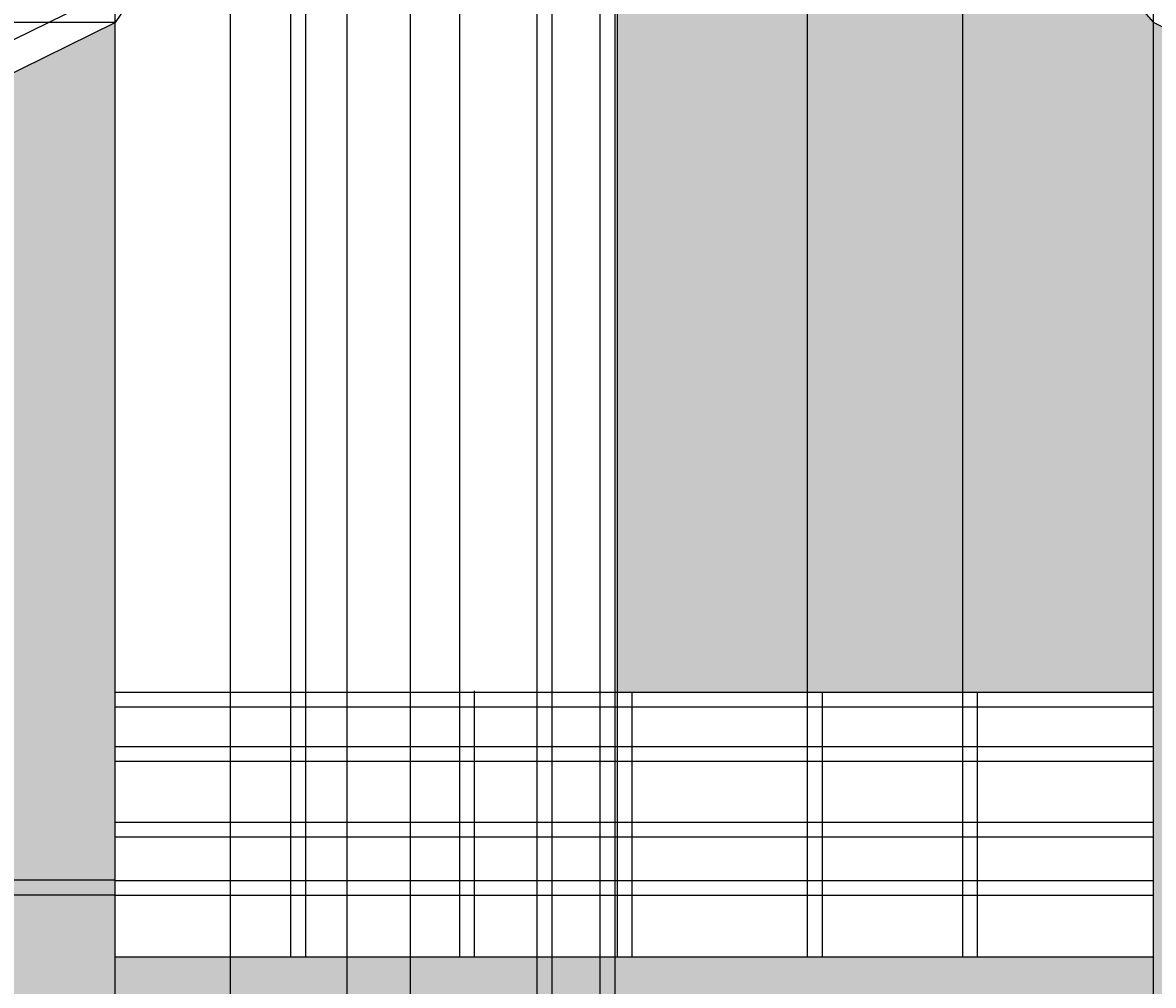
# Model space of a CAD drawing. Units: inches. Extents: x 36 to 594, y 79 to 831.
# Tile 23 of 30: x 189 to 342, y 590 to 721. Entities that reach past the tile are written whole.
import ezdxf

# ---------------------------------------------------------------- set-up
doc = ezdxf.new("R2010")
doc.units = ezdxf.units.IN
doc.header["$MEASUREMENT"] = 0
for name, color, linetype, lineweight in [('A-ANNO-DIMS', 2, 'Continuous', 18), ('A-ELEV', 7, 'Continuous', 25), ('A-ELEV-PATT', 8, 'Continuous', 13)]:
    doc.layers.add(name, color=color, linetype=linetype, lineweight=lineweight)
doc.styles.get("Standard").update_dxf_attribs({"font": 'arial.ttf'})
doc.dimstyles.get("Standard").update_dxf_attribs({"dimtxt": 0.8125, "dimasz": 0.18, "dimexe": 0.18, "dimexo": 0.0625, "dimgap": 0.09, "dimtad": 0, "dimtih": 1, "dimtoh": 1, "dimdec": 4, "dimzin": 0, "dimdsep": 46, "dimlunit": 4, "dimtxsty": 'Standard', "dimcen": 0.09, "dimadec": 0, "dimazin": 0, "dimtfac": 1, "dimtdec": 4, "dimtofl": 0, "dimtmove": 0, "dimatfit": 3, "dimfxl": 1, "dimtolj": 1, "dimtzin": 0, "dimarcsym": 0})

# ---------------------------------------------------------------- blocks, each defined once
blk = doc.blocks.new('*D14')
at = {"layer": 'A-ANNO-DIMS', "color": 0, "lineweight": -2, "transparency": 16777216}
for p, q in [((177.52, 594.27), (177.52, 830.73)), ((177.7, 830.55), (187.69, 830.55)), ((201.24, 830.55), (191.25, 830.55)), ((201.42, 720.66), (201.42, 830.73))]:
    blk.add_line(p, q, dxfattribs=at)
at = {"layer": 'A-ANNO-DIMS', "color": 0, "transparency": 16777216}
for points in [[(177.7, 830.58), (177.7, 830.52), (177.52, 830.55)], [(201.24, 830.58), (201.24, 830.52), (201.42, 830.55)]]:
    blk.add_solid(points, dxfattribs=at)
at = {"layer": 'Defpoints', "color": 0, "transparency": 16777216}
for p in [(201.42, 830.55), (201.42, 720.59), (177.52, 594.21)]:
    blk.add_point(p, dxfattribs=at)
at = {"layer": 'A-ANNO-DIMS', "color": 0, "transparency": 16777216, "insert": (189.47, 830.55), "char_height": 0.812, "attachment_point": 5}
blk.add_mtext('\\A1;23.894', dxfattribs=at)
blk = doc.blocks.new('*D28')
at = {"layer": 'A-ANNO-DIMS', "color": 0, "lineweight": -2, "transparency": 16777216}
for p, q in [((269.3, 796.05), (37.49, 796.05)), ((37.67, 795.87), (37.67, 455.63)), ((37.67, 114.39), (37.67, 454.62)), ((94.8, 114.21), (37.49, 114.21))]:
    blk.add_line(p, q, dxfattribs=at)
at = {"layer": 'A-ANNO-DIMS', "color": 0, "transparency": 16777216}
for points in [[(37.64, 795.87), (37.7, 795.87), (37.67, 796.05)], [(37.64, 114.39), (37.7, 114.39), (37.67, 114.21)]]:
    blk.add_solid(points, dxfattribs=at)
at = {"layer": 'Defpoints', "color": 0, "transparency": 16777216}
for p in [(37.67, 796.05), (269.36, 796.05), (94.87, 114.21)]:
    blk.add_point(p, dxfattribs=at)
at = {"layer": 'A-ANNO-DIMS', "color": 0, "transparency": 16777216, "insert": (37.67, 455.13), "char_height": 0.812, "attachment_point": 5}
blk.add_mtext('\\A1;681.8', dxfattribs=at)
blk = doc.blocks.new('*D37')
at = {"layer": 'A-ANNO-DIMS', "color": 0, "lineweight": -2, "transparency": 16777216}
for p, q in [((330.04, 735.34), (592.85, 735.34)), ((592.67, 735.16), (592.67, 702.28)), ((592.67, 668.39), (592.67, 701.27)), ((448.45, 668.21), (592.85, 668.21))]:
    blk.add_line(p, q, dxfattribs=at)
at = {"layer": 'A-ANNO-DIMS', "color": 0, "transparency": 16777216}
for points in [[(592.64, 735.16), (592.7, 735.16), (592.67, 735.34)], [(592.64, 668.39), (592.7, 668.39), (592.67, 668.21)]]:
    blk.add_solid(points, dxfattribs=at)
at = {"layer": 'Defpoints', "color": 0, "transparency": 16777216}
for p in [(329.98, 735.34), (592.67, 735.34), (448.39, 668.21)]:
    blk.add_point(p, dxfattribs=at)
at = {"layer": 'A-ANNO-DIMS', "color": 0, "transparency": 16777216, "insert": (592.67, 701.77), "char_height": 0.812, "attachment_point": 5}
blk.add_mtext('\\A1;67.12', dxfattribs=at)
blk = doc.blocks.new('*D48')
at = {"layer": 'A-ANNO-DIMS', "color": 0, "lineweight": -2, "transparency": 16777216}
for p, q in [((201.36, 720.59), (37.49, 720.59)), ((37.67, 720.41), (37.67, 694.91)), ((37.67, 668.39), (37.67, 693.9)), ((94.8, 668.21), (37.49, 668.21))]:
    blk.add_line(p, q, dxfattribs=at)
at = {"layer": 'A-ANNO-DIMS', "color": 0, "transparency": 16777216}
for points in [[(37.64, 720.41), (37.7, 720.41), (37.67, 720.59)], [(37.64, 668.39), (37.7, 668.39), (37.67, 668.21)]]:
    blk.add_solid(points, dxfattribs=at)
at = {"layer": 'Defpoints', "color": 0, "transparency": 16777216}
for p in [(37.67, 720.59), (201.42, 720.59), (94.87, 668.21)]:
    blk.add_point(p, dxfattribs=at)
at = {"layer": 'A-ANNO-DIMS', "color": 0, "transparency": 16777216, "insert": (37.67, 694.4), "char_height": 0.812, "attachment_point": 5}
blk.add_mtext('\\A1;52.38', dxfattribs=at)
blk = doc.blocks.new('*D61')
at = {"layer": 'A-ANNO-DIMS', "color": 0, "lineweight": -2, "transparency": 16777216}
for p, q in [((156.41, 264.68), (156.41, 830.73)), ((156.59, 830.55), (185.26, 830.55)), ((216.85, 830.55), (188.18, 830.55)), ((217.03, 286.24), (217.03, 830.73))]:
    blk.add_line(p, q, dxfattribs=at)
at = {"layer": 'A-ANNO-DIMS', "color": 0, "transparency": 16777216}
for points in [[(156.59, 830.58), (156.59, 830.52), (156.41, 830.55)], [(216.85, 830.58), (216.85, 830.52), (217.03, 830.55)]]:
    blk.add_solid(points, dxfattribs=at)
at = {"layer": 'Defpoints', "color": 0, "transparency": 16777216}
for p in [(217.03, 830.55), (217.03, 286.18), (156.41, 264.62)]:
    blk.add_point(p, dxfattribs=at)
at = {"layer": 'A-ANNO-DIMS', "color": 0, "transparency": 16777216, "insert": (186.72, 830.55), "char_height": 0.812, "attachment_point": 5}
blk.add_mtext('\\A1;60.62', dxfattribs=at)
blk = doc.blocks.new('*D92')
at = {"layer": 'A-ANNO-DIMS', "color": 0, "lineweight": -2, "transparency": 16777216}
for p, q in [((201.42, 475.48), (201.42, 830.73)), ((201.6, 830.55), (215.98, 830.55)), ((232.64, 830.55), (218.26, 830.55)), ((232.82, 524.67), (232.82, 830.73))]:
    blk.add_line(p, q, dxfattribs=at)
at = {"layer": 'A-ANNO-DIMS', "color": 0, "transparency": 16777216}
for points in [[(201.6, 830.58), (201.6, 830.52), (201.42, 830.55)], [(232.64, 830.58), (232.64, 830.52), (232.82, 830.55)]]:
    blk.add_solid(points, dxfattribs=at)
at = {"layer": 'Defpoints', "color": 0, "transparency": 16777216}
for p in [(232.82, 830.55), (232.82, 524.6), (201.42, 475.41)]:
    blk.add_point(p, dxfattribs=at)
at = {"layer": 'A-ANNO-DIMS', "color": 0, "transparency": 16777216, "insert": (217.12, 830.55), "char_height": 0.812, "attachment_point": 5}
blk.add_mtext('\\A1;31.4', dxfattribs=at)
blk = doc.blocks.new('*D93')
at = {"layer": 'A-ANNO-DIMS', "color": 0, "lineweight": -2, "transparency": 16777216}
for p, q in [((232.82, 524.67), (232.82, 830.73)), ((233, 830.55), (243.88, 830.55)), ((258.33, 830.55), (247.45, 830.55)), ((258.51, 524.67), (258.51, 830.73))]:
    blk.add_line(p, q, dxfattribs=at)
at = {"layer": 'A-ANNO-DIMS', "color": 0, "transparency": 16777216}
for points in [[(233, 830.58), (233, 830.52), (232.82, 830.55)], [(258.33, 830.58), (258.33, 830.52), (258.51, 830.55)]]:
    blk.add_solid(points, dxfattribs=at)
at = {"layer": 'Defpoints', "color": 0, "transparency": 16777216}
for p in [(258.51, 830.55), (232.82, 524.6), (258.51, 524.6)]:
    blk.add_point(p, dxfattribs=at)
at = {"layer": 'A-ANNO-DIMS', "color": 0, "transparency": 16777216, "insert": (245.66, 830.55), "char_height": 0.812, "attachment_point": 5}
blk.add_mtext('\\A1;25.684', dxfattribs=at)
blk = doc.blocks.new('*D94')
at = {"layer": 'A-ANNO-DIMS', "color": 0, "lineweight": -2, "transparency": 16777216}
for p, q in [((258.51, 524.67), (258.51, 830.73)), ((258.69, 830.55), (259.15, 830.55)), ((260.33, 830.55), (259.86, 830.55)), ((260.51, 524.67), (260.51, 830.73))]:
    blk.add_line(p, q, dxfattribs=at)
at = {"layer": 'A-ANNO-DIMS', "color": 0, "transparency": 16777216}
for points in [[(258.69, 830.58), (258.69, 830.52), (258.51, 830.55)], [(260.33, 830.58), (260.33, 830.52), (260.51, 830.55)]]:
    blk.add_solid(points, dxfattribs=at)
at = {"layer": 'Defpoints', "color": 0, "transparency": 16777216}
for p in [(260.51, 830.55), (258.51, 524.6), (260.51, 524.6)]:
    blk.add_point(p, dxfattribs=at)
at = {"layer": 'A-ANNO-DIMS', "color": 0, "transparency": 16777216, "insert": (259.51, 830.55), "char_height": 0.812, "attachment_point": 5}
blk.add_mtext('\\A1;2', dxfattribs=at)
blk = doc.blocks.new('*D95')
at = {"layer": 'A-ANNO-DIMS', "color": 0, "lineweight": -2, "transparency": 16777216}
for p, q in [((260.51, 524.67), (260.51, 830.73)), ((260.69, 830.55), (299.71, 830.55)), ((341.66, 830.55), (302.63, 830.55)), ((341.84, 524.67), (341.84, 830.73))]:
    blk.add_line(p, q, dxfattribs=at)
at = {"layer": 'A-ANNO-DIMS', "color": 0, "transparency": 16777216}
for points in [[(260.69, 830.58), (260.69, 830.52), (260.51, 830.55)], [(341.66, 830.58), (341.66, 830.52), (341.84, 830.55)]]:
    blk.add_solid(points, dxfattribs=at)
at = {"layer": 'Defpoints', "color": 0, "transparency": 16777216}
for p in [(341.84, 830.55), (260.51, 524.6), (341.84, 524.6)]:
    blk.add_point(p, dxfattribs=at)
at = {"layer": 'A-ANNO-DIMS', "color": 0, "transparency": 16777216, "insert": (301.17, 830.55), "char_height": 0.812, "attachment_point": 5}
blk.add_mtext('\\A1;81.33', dxfattribs=at)
blk = doc.blocks.new('*D105')
at = {"layer": 'A-ANNO-DIMS', "color": 0, "lineweight": -2, "transparency": 16777216}
for p, q in [((241.36, 404.34), (241.36, 830.73)), ((241.54, 830.55), (252.42, 830.55)), ((266.86, 830.55), (255.98, 830.55)), ((267.04, 404.34), (267.04, 830.73))]:
    blk.add_line(p, q, dxfattribs=at)
at = {"layer": 'A-ANNO-DIMS', "color": 0, "transparency": 16777216}
for points in [[(241.54, 830.58), (241.54, 830.52), (241.36, 830.55)], [(266.86, 830.58), (266.86, 830.52), (267.04, 830.55)]]:
    blk.add_solid(points, dxfattribs=at)
at = {"layer": 'Defpoints', "color": 0, "transparency": 16777216}
for p in [(267.04, 830.55), (241.36, 404.27), (267.04, 404.27)]:
    blk.add_point(p, dxfattribs=at)
at = {"layer": 'A-ANNO-DIMS', "color": 0, "transparency": 16777216, "insert": (254.2, 830.55), "char_height": 0.812, "attachment_point": 5}
blk.add_mtext('\\A1;25.684', dxfattribs=at)
blk = doc.blocks.new('*D106')
at = {"layer": 'A-ANNO-DIMS', "color": 0, "lineweight": -2, "transparency": 16777216}
for p, q in [((267.04, 404.34), (267.04, 830.73)), ((267.22, 830.55), (267.68, 830.55)), ((268.86, 830.55), (268.4, 830.55)), ((269.04, 404.34), (269.04, 830.73))]:
    blk.add_line(p, q, dxfattribs=at)
at = {"layer": 'A-ANNO-DIMS', "color": 0, "transparency": 16777216}
for points in [[(267.22, 830.58), (267.22, 830.52), (267.04, 830.55)], [(268.86, 830.58), (268.86, 830.52), (269.04, 830.55)]]:
    blk.add_solid(points, dxfattribs=at)
at = {"layer": 'Defpoints', "color": 0, "transparency": 16777216}
for p in [(269.04, 830.55), (267.04, 404.27), (269.04, 404.27)]:
    blk.add_point(p, dxfattribs=at)
at = {"layer": 'A-ANNO-DIMS', "color": 0, "transparency": 16777216, "insert": (268.04, 830.55), "char_height": 0.812, "attachment_point": 5}
blk.add_mtext('\\A1;2', dxfattribs=at)
blk = doc.blocks.new('*D107')
at = {"layer": 'A-ANNO-DIMS', "color": 0, "lineweight": -2, "transparency": 16777216}
for p, q in [((269.04, 404.34), (269.04, 830.73)), ((269.22, 830.55), (310.99, 830.55)), ((355.68, 830.55), (313.91, 830.55)), ((355.86, 404.34), (355.86, 830.73))]:
    blk.add_line(p, q, dxfattribs=at)
at = {"layer": 'A-ANNO-DIMS', "color": 0, "transparency": 16777216}
for points in [[(269.22, 830.58), (269.22, 830.52), (269.04, 830.55)], [(355.68, 830.58), (355.68, 830.52), (355.86, 830.55)]]:
    blk.add_solid(points, dxfattribs=at)
at = {"layer": 'Defpoints', "color": 0, "transparency": 16777216}
for p in [(355.86, 830.55), (269.04, 404.27), (355.86, 404.27)]:
    blk.add_point(p, dxfattribs=at)
at = {"layer": 'A-ANNO-DIMS', "color": 0, "transparency": 16777216, "insert": (312.45, 830.55), "char_height": 0.812, "attachment_point": 5}
blk.add_mtext('\\A1;86.82', dxfattribs=at)
blk = doc.blocks.new('*D122')
at = {"layer": 'A-ANNO-DIMS', "color": 0, "lineweight": -2, "transparency": 16777216}
for p, q in [((201.36, 604.57), (37.49, 604.57)), ((37.67, 604.39), (37.67, 604.06)), ((201.36, 602.57), (37.49, 602.57)), ((37.67, 602.75), (37.67, 603.07))]:
    blk.add_line(p, q, dxfattribs=at)
at = {"layer": 'A-ANNO-DIMS', "color": 0, "transparency": 16777216}
for points in [[(37.64, 604.39), (37.7, 604.39), (37.67, 604.57)], [(37.64, 602.75), (37.7, 602.75), (37.67, 602.57)]]:
    blk.add_solid(points, dxfattribs=at)
at = {"layer": 'Defpoints', "color": 0, "transparency": 16777216}
for p in [(37.67, 604.57), (201.42, 604.57), (201.42, 602.57)]:
    blk.add_point(p, dxfattribs=at)
at = {"layer": 'A-ANNO-DIMS', "color": 0, "transparency": 16777216, "insert": (37.67, 603.57), "char_height": 0.812, "attachment_point": 5}
blk.add_mtext('\\A1;2', dxfattribs=at)
blk = doc.blocks.new('*D123')
at = {"layer": 'A-ANNO-DIMS', "color": 0, "lineweight": -2, "transparency": 16777216}
for p, q in [((201.42, 630.1), (201.42, 830.73)), ((201.6, 830.55), (211.52, 830.55)), ((225.01, 830.55), (215.09, 830.55)), ((225.19, 630.1), (225.19, 830.73))]:
    blk.add_line(p, q, dxfattribs=at)
at = {"layer": 'A-ANNO-DIMS', "color": 0, "transparency": 16777216}
for points in [[(201.6, 830.58), (201.6, 830.52), (201.42, 830.55)], [(225.01, 830.58), (225.01, 830.52), (225.19, 830.55)]]:
    blk.add_solid(points, dxfattribs=at)
at = {"layer": 'Defpoints', "color": 0, "transparency": 16777216}
for p in [(225.19, 830.55), (201.42, 630.04), (225.19, 630.04)]:
    blk.add_point(p, dxfattribs=at)
at = {"layer": 'A-ANNO-DIMS', "color": 0, "transparency": 16777216, "insert": (213.31, 830.55), "char_height": 0.812, "attachment_point": 5}
blk.add_mtext('\\A1;23.773', dxfattribs=at)
blk = doc.blocks.new('*D124')
at = {"layer": 'A-ANNO-DIMS', "color": 0, "lineweight": -2, "transparency": 16777216}
for p, q in [((225.19, 630.1), (225.19, 830.73)), ((225.37, 830.55), (225.83, 830.55)), ((227.01, 830.55), (226.55, 830.55)), ((227.19, 630.1), (227.19, 830.73))]:
    blk.add_line(p, q, dxfattribs=at)
at = {"layer": 'A-ANNO-DIMS', "color": 0, "transparency": 16777216}
for points in [[(225.37, 830.58), (225.37, 830.52), (225.19, 830.55)], [(227.01, 830.58), (227.01, 830.52), (227.19, 830.55)]]:
    blk.add_solid(points, dxfattribs=at)
at = {"layer": 'Defpoints', "color": 0, "transparency": 16777216}
for p in [(227.19, 830.55), (225.19, 630.04), (227.19, 630.04)]:
    blk.add_point(p, dxfattribs=at)
at = {"layer": 'A-ANNO-DIMS', "color": 0, "transparency": 16777216, "insert": (226.19, 830.55), "char_height": 0.812, "attachment_point": 5}
blk.add_mtext('\\A1;2', dxfattribs=at)
blk = doc.blocks.new('*D125')
at = {"layer": 'A-ANNO-DIMS', "color": 0, "lineweight": -2, "transparency": 16777216}
for p, q in [((227.19, 630.1), (227.19, 830.73)), ((227.37, 830.55), (236.14, 830.55)), ((247.84, 830.55), (239.07, 830.55)), ((248.02, 630.27), (248.02, 830.73))]:
    blk.add_line(p, q, dxfattribs=at)
at = {"layer": 'A-ANNO-DIMS', "color": 0, "transparency": 16777216}
for points in [[(227.37, 830.58), (227.37, 830.52), (227.19, 830.55)], [(247.84, 830.58), (247.84, 830.52), (248.02, 830.55)]]:
    blk.add_solid(points, dxfattribs=at)
at = {"layer": 'Defpoints', "color": 0, "transparency": 16777216}
for p in [(248.02, 830.55), (248.02, 630.21), (227.19, 630.04)]:
    blk.add_point(p, dxfattribs=at)
at = {"layer": 'A-ANNO-DIMS', "color": 0, "transparency": 16777216, "insert": (237.61, 830.55), "char_height": 0.812, "attachment_point": 5}
blk.add_mtext('\\A1;20.83', dxfattribs=at)
blk = doc.blocks.new('*D126')
at = {"layer": 'A-ANNO-DIMS', "color": 0, "lineweight": -2, "transparency": 16777216}
for p, q in [((248.02, 630.27), (248.02, 830.73)), ((248.2, 830.55), (256.91, 830.55)), ((269.18, 830.55), (260.47, 830.55)), ((269.36, 630.1), (269.36, 830.73))]:
    blk.add_line(p, q, dxfattribs=at)
at = {"layer": 'A-ANNO-DIMS', "color": 0, "transparency": 16777216}
for points in [[(248.2, 830.58), (248.2, 830.52), (248.02, 830.55)], [(269.18, 830.58), (269.18, 830.52), (269.36, 830.55)]]:
    blk.add_solid(points, dxfattribs=at)
at = {"layer": 'Defpoints', "color": 0, "transparency": 16777216}
for p in [(269.36, 830.55), (248.02, 630.21), (269.36, 630.04)]:
    blk.add_point(p, dxfattribs=at)
at = {"layer": 'A-ANNO-DIMS', "color": 0, "transparency": 16777216, "insert": (258.69, 830.55), "char_height": 0.812, "attachment_point": 5}
blk.add_mtext('\\A1;21.338', dxfattribs=at)
blk = doc.blocks.new('*D127')
at = {"layer": 'A-ANNO-DIMS', "color": 0, "lineweight": -2, "transparency": 16777216}
for p, q in [((269.36, 630.1), (269.36, 830.73)), ((269.54, 830.55), (280.75, 830.55)), ((294.9, 830.55), (283.68, 830.55)), ((295.08, 630.1), (295.08, 830.73))]:
    blk.add_line(p, q, dxfattribs=at)
at = {"layer": 'A-ANNO-DIMS', "color": 0, "transparency": 16777216}
for points in [[(269.54, 830.58), (269.54, 830.52), (269.36, 830.55)], [(294.9, 830.58), (294.9, 830.52), (295.08, 830.55)]]:
    blk.add_solid(points, dxfattribs=at)
at = {"layer": 'Defpoints', "color": 0, "transparency": 16777216}
for p in [(295.08, 830.55), (269.36, 630.04), (295.08, 630.04)]:
    blk.add_point(p, dxfattribs=at)
at = {"layer": 'A-ANNO-DIMS', "color": 0, "transparency": 16777216, "insert": (282.22, 830.55), "char_height": 0.812, "attachment_point": 5}
blk.add_mtext('\\A1;25.72', dxfattribs=at)
blk = doc.blocks.new('*D128')
at = {"layer": 'A-ANNO-DIMS', "color": 0, "lineweight": -2, "transparency": 16777216}
for p, q in [((295.08, 630.1), (295.08, 830.73)), ((295.26, 830.55), (303.78, 830.55)), ((315.87, 830.55), (307.35, 830.55)), ((316.05, 630.1), (316.05, 830.73))]:
    blk.add_line(p, q, dxfattribs=at)
at = {"layer": 'A-ANNO-DIMS', "color": 0, "transparency": 16777216}
for points in [[(295.26, 830.58), (295.26, 830.52), (295.08, 830.55)], [(315.87, 830.58), (315.87, 830.52), (316.05, 830.55)]]:
    blk.add_solid(points, dxfattribs=at)
at = {"layer": 'Defpoints', "color": 0, "transparency": 16777216}
for p in [(316.05, 830.55), (295.08, 630.04), (316.05, 630.04)]:
    blk.add_point(p, dxfattribs=at)
at = {"layer": 'A-ANNO-DIMS', "color": 0, "transparency": 16777216, "insert": (305.56, 830.55), "char_height": 0.812, "attachment_point": 5}
blk.add_mtext('\\A1;20.974', dxfattribs=at)
blk = doc.blocks.new('*D129')
at = {"layer": 'A-ANNO-DIMS', "color": 0, "lineweight": -2, "transparency": 16777216}
for p, q in [((316.05, 630.1), (316.05, 830.73)), ((316.23, 830.55), (327.16, 830.55)), ((341.66, 830.55), (330.73, 830.55)), ((341.84, 630.1), (341.84, 830.73))]:
    blk.add_line(p, q, dxfattribs=at)
at = {"layer": 'A-ANNO-DIMS', "color": 0, "transparency": 16777216}
for points in [[(316.23, 830.58), (316.23, 830.52), (316.05, 830.55)], [(341.66, 830.58), (341.66, 830.52), (341.84, 830.55)]]:
    blk.add_solid(points, dxfattribs=at)
at = {"layer": 'Defpoints', "color": 0, "transparency": 16777216}
for p in [(341.84, 830.55), (316.05, 630.04), (341.84, 630.04)]:
    blk.add_point(p, dxfattribs=at)
at = {"layer": 'A-ANNO-DIMS', "color": 0, "transparency": 16777216, "insert": (328.94, 830.55), "char_height": 0.812, "attachment_point": 5}
blk.add_mtext('\\A1;25.785', dxfattribs=at)

msp = doc.modelspace()

# ---------------------------------------------------------------- hatches: boundary and pattern name
at = {"layer": 'A-ELEV-PATT'}
h = msp.add_hatch(color=256, dxfattribs=at)
h.dxf.hatch_style = 1
h.paths.add_polyline_path([(398.0873, 796.0465), (269.3592, 796.0465), (269.3592, 770.1455), (397.8159, 770.1455)])
h.paths.add_polyline_path([(397.7518, 764.0341), (269.3592, 764.0341), (269.3592, 630.0394), (341.8367, 630.0394), (341.8367, 720.595), (335.0881, 728.3699), (329.982, 735.3373), (345.3661, 727.7743), (397.1052, 702.3389)])
h.paths.add_polyline_path([(341.8367, 594.2124), (201.4189, 594.2124), (201.4189, 475.4136), (232.8216, 475.4136), (232.8216, 524.6037), (341.8367, 524.6037)])
h.paths.add_polyline_path([(177.525, 594.2124), (118.7598, 594.2124), (118.7598, 450.2124), (177.525, 450.2124)])
h.paths.add_polyline_path([(424.4958, 594.2124), (365.7306, 594.2124), (365.7306, 450.2124), (424.4958, 450.2124)])
h.paths.add_polyline_path([(241.3553, 404.2737), (355.8569, 404.2737), (355.8569, 355.0836), (424.5492, 355.0836), (424.5492, 425.7333), (118.7598, 426.2844), (118.7598, 355.0836), (241.3553, 355.0836)])
h.paths.add_polyline_path([(448.3898, 306.2124), (217.0273, 306.2124), (217.0273, 142.2124), (254.0293, 142.2124), (254.0293, 150.9347), (254.0293, 286.1802), (401.5491, 286.1802), (401.5491, 150.9347), (401.5491, 142.2124), (448.3898, 142.2124)])
h.paths.add_polyline_path([(448.3898, 142.2124), (401.5491, 142.2124), (217.0273, 142.2124), (217.0273, 114.2124), (448.3898, 114.2124)])
h.paths.add_polyline_path([(217.0273, 306.2124), (174.7353, 306.2124), (94.8658, 306.2124), (94.8658, 162.2124), (103.3368, 162.2124), (103.3368, 264.6224), (103.3368, 286.1802), (217.0273, 286.1802)])
h = msp.add_hatch(color=256, dxfattribs=at)
h.dxf.hatch_style = 1
h.paths.add_polyline_path([(448.3898, 668.2124), (341.8367, 720.595), (341.8367, 594.2124), (341.8367, 450.2124), (365.7306, 450.2124), (365.7306, 594.2124), (424.4958, 594.2124), (424.4958, 450.2124), (448.3898, 450.2124), (448.3898, 594.2124)])
h.paths.add_polyline_path([(378.5958, 653.8563, -1), (413.2033, 653.8563, -1)], flags=16)
h.paths.add_polyline_path([(394.8995, 653.8563), (394.8995, 654.8563), (395.8995, 654.8563), (396.8995, 654.8563), (396.8995, 653.8563), (396.8995, 652.8563), (395.8995, 652.8563), (394.8995, 652.8563)], flags=0)
h.paths.add_polyline_path([(201.4189, 708.8485), (201.4189, 720.595), (94.8658, 668.2124), (94.8658, 644.2124), (94.8658, 596.2124), (94.8658, 594.2124), (94.8658, 450.2124), (118.7598, 450.2124), (118.7598, 594.2124), (177.525, 594.2124), (177.525, 450.2124), (201.4189, 450.2124), (201.4189, 594.2124)])
h.paths.add_polyline_path([(130.1589, 653.7648, -1), (164.7665, 653.7648, -1)], flags=16)
h.paths.add_polyline_path([(148.4627, 652.7648), (147.4627, 652.7648), (146.4627, 652.7648), (146.4627, 653.7648), (146.4627, 654.7648), (147.4627, 654.7648), (148.4627, 654.7648), (148.4627, 653.7648)], flags=0)

# ---------------------------------------------------------------- linework, layer by layer
at = {"layer": 'A-ELEV'}
for p, q in [((269.3592, 630.0394), (269.3592, 796.0465)), ((335.0881, 728.3699), (341.8367, 720.595)), ((205.9095, 727.2598), (201.4189, 720.595)), ((93.1011, 671.802), (199.6542, 724.1846)), ((94.8658, 668.2124), (201.4189, 720.595)), ((201.4189, 708.8485), (201.4189, 720.595)), ((341.8367, 594.2124), (341.8367, 720.595)), ((448.3898, 668.2124), (341.8367, 720.595)), ((201.4189, 594.2124), (201.4189, 708.8485)), ((248.0217, 594.2124), (248.0217, 630.2124)), ((250.0217, 594.2124), (250.0217, 630.2124)), ((201.4189, 630.0394), (341.8367, 630.0394)), ((225.1915, 594.2124), (225.1915, 630.0394)), ((227.1915, 594.2124), (227.1915, 630.0394)), ((269.3592, 594.2124), (269.3592, 630.0394)), ((271.3592, 594.2124), (271.3592, 630.0394)), ((295.0778, 594.2124), (295.0778, 630.0394)), ((297.0778, 594.2124), (297.0778, 630.0394)), ((316.0513, 594.2124), (316.0513, 630.0394)), ((318.0513, 594.2124), (318.0513, 630.0394)), ((201.4189, 628.0394), (341.8367, 628.0394)), ((201.4189, 622.6866), (341.8367, 622.6866)), ((201.4189, 620.6866), (341.8367, 620.6866)), ((201.4189, 612.4402), (341.8367, 612.4402)), ((201.4189, 610.4402), (341.8367, 610.4402)), ((201.4189, 604.5667), (341.8367, 604.5667)), ((201.4189, 602.5667), (341.8367, 602.5667)), ((201.4189, 450.2124), (201.4189, 594.2124)), ((201.4189, 594.2124), (341.8367, 594.2124)), ((341.8367, 450.2124), (341.8367, 594.2124))]:
    msp.add_line(p, q, dxfattribs=at)

# ---------------------------------------------------------------- dimensions: what is measured, and where the dimension line sits
at = {"layer": 'A-ANNO-DIMS'}
for base, p1, p2, override, picture, middle in [((217.0273, 830.5465), (156.4069, 264.6224), (217.0273, 286.1802), {"dimdec": 2, "dimlfac": 1, "dimrnd": 0, "dimzin": 0, "dimdsep": 46, "dimlunit": 2}, '*D61', (186.7171, 830.5465)), ((201.4189, 830.5465), (177.525, 594.2124), (201.4189, 720.595), {"dimdec": 3, "dimlfac": 1, "dimrnd": 0, "dimzin": 0, "dimdsep": 46, "dimlunit": 2}, '*D14', (189.4719, 830.5465)), ((232.8216, 830.5465), (201.4189, 475.4136), (232.8216, 524.6037), {"dimdec": 1, "dimlfac": 1, "dimrnd": 0, "dimzin": 0, "dimdsep": 46, "dimlunit": 2}, '*D92', (217.1202, 830.5465)), ((225.1915, 830.5465), (201.4189, 630.0394), (225.1915, 630.0394), {"dimdec": 3, "dimlfac": 1, "dimrnd": 0, "dimzin": 0, "dimdsep": 46, "dimlunit": 2}, '*D123', (213.3052, 830.5465)), ((227.1915, 830.5465), (225.1915, 630.0394), (227.1915, 630.0394), {"dimdec": 0, "dimlfac": 1, "dimrnd": 0, "dimzin": 0, "dimdsep": 46, "dimlunit": 2}, '*D124', (226.1915, 830.5465)), ((248.0217, 830.5465), (227.1915, 630.0394), (248.0217, 630.2124), {"dimdec": 2, "dimlfac": 1, "dimrnd": 0, "dimzin": 0, "dimdsep": 46, "dimlunit": 2}, '*D125', (237.6066, 830.5465)), ((258.5056, 830.5465), (232.8216, 524.6037), (258.5056, 524.6037), {"dimdec": 3, "dimlfac": 1, "dimrnd": 0, "dimzin": 0, "dimdsep": 46, "dimlunit": 2}, '*D93', (245.6636, 830.5465)), ((267.0393, 830.5465), (241.3553, 404.2737), (267.0393, 404.2737), {"dimdec": 3, "dimlfac": 1, "dimrnd": 0, "dimzin": 0, "dimdsep": 46, "dimlunit": 2}, '*D105', (254.1973, 830.5465)), ((269.35917, 830.54647), (248.02166, 630.21236), (269.35917, 630.03937), {"dimdec": 3, "dimlfac": 1, "dimrnd": 0, "dimzin": 0, "dimdsep": 46, "dimlunit": 2}, '*D126', (258.69041, 830.54647)), ((260.5056, 830.5465), (258.5056, 524.6037), (260.5056, 524.6037), {"dimdec": 0, "dimlfac": 1, "dimrnd": 0, "dimzin": 0, "dimdsep": 46, "dimlunit": 2}, '*D94', (259.5056, 830.5465)), ((341.8367, 830.5465), (260.5056, 524.6037), (341.8367, 524.6037), {"dimdec": 2, "dimlfac": 1, "dimrnd": 0, "dimzin": 0, "dimdsep": 46, "dimlunit": 2}, '*D95', (301.1711, 830.5465)), ((269.0393, 830.5465), (267.0393, 404.2737), (269.0393, 404.2737), {"dimdec": 0, "dimlfac": 1, "dimrnd": 0, "dimzin": 0, "dimdsep": 46, "dimlunit": 2}, '*D106', (268.0393, 830.5465)), ((355.8569, 830.5465), (269.0393, 404.2737), (355.8569, 404.2737), {"dimdec": 2, "dimlfac": 1, "dimrnd": 0, "dimzin": 0, "dimdsep": 46, "dimlunit": 2}, '*D107', (312.4481, 830.5465)), ((295.0778, 830.5465), (269.3592, 630.0394), (295.0778, 630.0394), {"dimdec": 2, "dimlfac": 1, "dimrnd": 0, "dimzin": 0, "dimdsep": 46, "dimlunit": 2}, '*D127', (282.2185, 830.5465)), ((316.0513, 830.54647), (295.07777, 630.03937), (316.0513, 630.03937), {"dimdec": 3, "dimlfac": 1, "dimrnd": 0, "dimzin": 0, "dimdsep": 46, "dimlunit": 2}, '*D128', (305.56454, 830.54647)), ((341.8367, 830.5465), (316.0513, 630.0394), (341.8367, 630.0394), {"dimdec": 3, "dimlfac": 1, "dimrnd": 0, "dimzin": 0, "dimdsep": 46, "dimlunit": 2}, '*D129', (328.944, 830.5465))]:
    dim = msp.add_linear_dim(base=base, p1=p1, p2=p2, dimstyle='Standard', override=override, dxfattribs=at)
    dim.commit()
    dim.dimension.update_dxf_attribs({"geometry": picture, "text_midpoint": middle})
for base, p1, p2, override, picture, middle in [((37.6733, 796.0465), (94.8658, 114.2124), (269.3592, 796.0465), {"dimdec": 1, "dimlfac": 1, "dimrnd": 0, "dimzin": 0, "dimdsep": 46, "dimlunit": 2}, '*D28', (37.6733, 455.1294)), ((592.6689, 735.3373), (448.3898, 668.2124), (329.982, 735.3373), {"dimdec": 2, "dimlfac": 1, "dimrnd": 0, "dimzin": 0, "dimdsep": 46, "dimlunit": 2}, '*D37', (592.6689, 701.7748)), ((37.6733, 720.595), (94.8658, 668.2124), (201.4189, 720.595), {"dimdec": 2, "dimlfac": 1, "dimrnd": 0, "dimzin": 0, "dimdsep": 46, "dimlunit": 2}, '*D48', (37.6733, 694.4037)), ((37.6733, 604.5667), (201.4189, 602.5667), (201.4189, 604.5667), {"dimdec": 0, "dimlfac": 1, "dimrnd": 0, "dimzin": 0, "dimdsep": 46, "dimlunit": 2}, '*D122', (37.6733, 603.5667))]:
    dim = msp.add_linear_dim(base=base, p1=p1, p2=p2, angle=90, dimstyle='Standard', override=override, dxfattribs=at)
    dim.commit()
    dim.dimension.update_dxf_attribs({"geometry": picture, "text_midpoint": middle})

doc.saveas('drawing.dxf')
